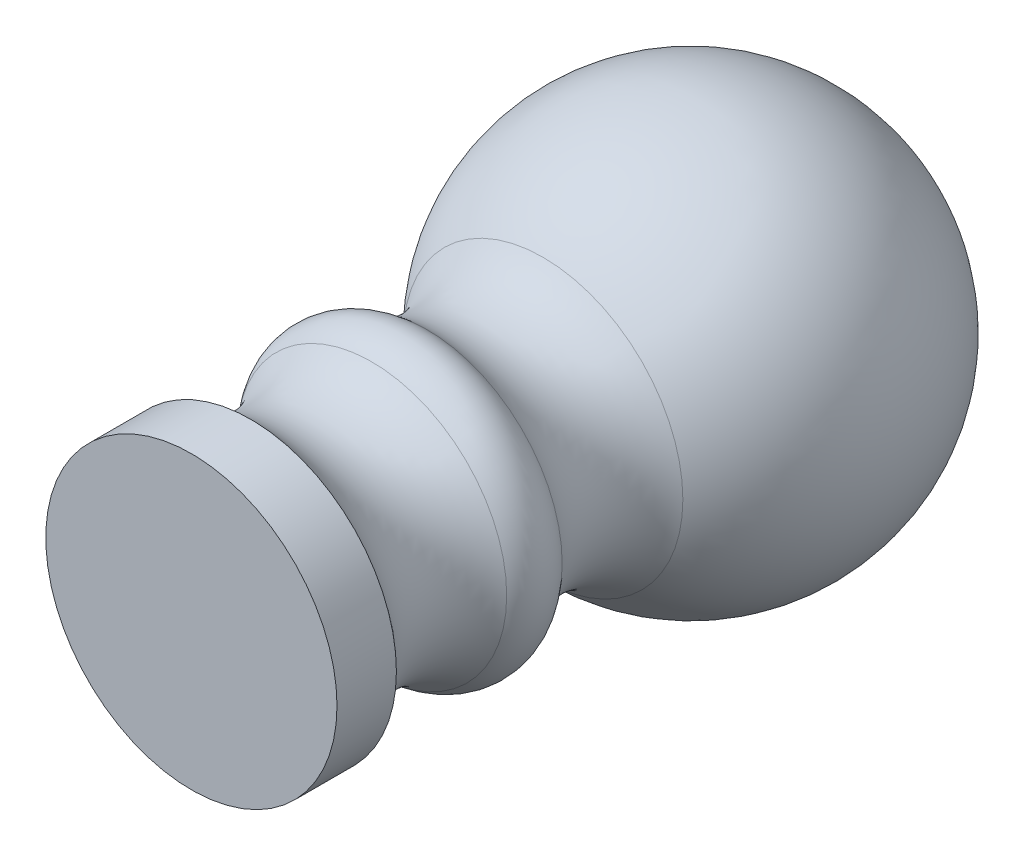
ISO-10303-21;
HEADER;
FILE_DESCRIPTION(('STEP AP214'),'2;1');
FILE_NAME('part.step','',(''),(''),'','','');
FILE_SCHEMA(('AUTOMOTIVE_DESIGN { 1 0 10303 214 1 1 1 1 }'));
ENDSEC;
DATA;
#1=APPLICATION_CONTEXT('core data for automotive mechanical design processes');
#2=APPLICATION_PROTOCOL_DEFINITION('international standard','automotive_design',2000,#1);
#3=PRODUCT_CONTEXT('',#1,'mechanical');
#4=PRODUCT('Part','Part','',(#3));
#5=PRODUCT_RELATED_PRODUCT_CATEGORY('part','',(#4));
#6=PRODUCT_DEFINITION_FORMATION('','',#4);
#7=PRODUCT_DEFINITION_CONTEXT('part definition',#1,'design');
#8=PRODUCT_DEFINITION('design','',#6,#7);
#9=PRODUCT_DEFINITION_SHAPE('','',#8);
#10=(LENGTH_UNIT() NAMED_UNIT(*) SI_UNIT(.MILLI.,.METRE.));
#11=(NAMED_UNIT(*) PLANE_ANGLE_UNIT() SI_UNIT($,.RADIAN.));
#12=(NAMED_UNIT(*) SI_UNIT($,.STERADIAN.) SOLID_ANGLE_UNIT());
#13=UNCERTAINTY_MEASURE_WITH_UNIT(LENGTH_MEASURE(1.E-05),#10,'distance_accuracy_value','');
#14=(GEOMETRIC_REPRESENTATION_CONTEXT(3) GLOBAL_UNCERTAINTY_ASSIGNED_CONTEXT((#13)) GLOBAL_UNIT_ASSIGNED_CONTEXT((#10,
#11,#12)) REPRESENTATION_CONTEXT('',''));
#15=CARTESIAN_POINT('',(0.,0.,0.));
#16=DIRECTION('',(0.,0.,1.));
#17=DIRECTION('',(1.,0.,0.));
#18=AXIS2_PLACEMENT_3D('',#15,#16,#17);
#19=CARTESIAN_POINT('',(0.,0.,-24.));
#20=DIRECTION('',(0.,0.,1.));
#21=DIRECTION('',(1.,0.,0.));
#22=AXIS2_PLACEMENT_3D('',#19,#20,#21);
#23=SPHERICAL_SURFACE('',#22,9.77393769225038);
#24=CARTESIAN_POINT('',(-8.91795144705289,0.,-24.));
#25=DIRECTION('',(1.,0.,0.));
#26=DIRECTION('',(0.,0.,-1.));
#27=AXIS2_PLACEMENT_3D('',#24,#25,#26);
#28=CIRCLE('',#27,4.);
#29=CARTESIAN_POINT('',(-8.91795144705289,0.,-28.));
#30=VERTEX_POINT('',#29);
#31=EDGE_CURVE('E45',#30,#30,#28,.T.);
#32=ORIENTED_EDGE('',*,*,#31,.T.);
#33=EDGE_LOOP('',(#32));
#34=FACE_BOUND('',#33,.T.);
#35=CARTESIAN_POINT('',(0.,0.,-16.9040352071946));
#36=DIRECTION('',(0.,0.,1.));
#37=DIRECTION('',(1.,0.,0.));
#38=AXIS2_PLACEMENT_3D('',#35,#36,#37);
#39=CIRCLE('',#38,6.72139432493431);
#40=CARTESIAN_POINT('',(6.72139432493431,0.,-16.9040352071946));
#41=VERTEX_POINT('',#40);
#42=EDGE_CURVE('E106',#41,#41,#39,.T.);
#43=ORIENTED_EDGE('',*,*,#42,.F.);
#44=EDGE_LOOP('',(#43));
#45=FACE_BOUND('',#44,.T.);
#46=CARTESIAN_POINT('',(0.,-8.91795144705289,-24.));
#47=DIRECTION('',(0.,1.,0.));
#48=DIRECTION('',(0.,0.,1.));
#49=AXIS2_PLACEMENT_3D('',#46,#47,#48);
#50=CIRCLE('',#49,4.);
#51=CARTESIAN_POINT('',(0.,-8.91795144705289,-20.));
#52=VERTEX_POINT('',#51);
#53=EDGE_CURVE('E100',#52,#52,#50,.T.);
#54=ORIENTED_EDGE('',*,*,#53,.T.);
#55=EDGE_LOOP('',(#54));
#56=FACE_BOUND('',#55,.T.);
#57=ADVANCED_FACE('F39',(#34,#45,#56),#23,.T.);
#58=CARTESIAN_POINT('',(4.,0.,-24.));
#59=DIRECTION('',(-1.,0.,0.));
#60=DIRECTION('',(0.,0.,1.));
#61=AXIS2_PLACEMENT_3D('',#58,#59,#60);
#62=CYLINDRICAL_SURFACE('',#61,4.);
#63=ORIENTED_EDGE('',*,*,#31,.F.);
#64=EDGE_LOOP('',(#63));
#65=FACE_BOUND('',#64,.T.);
#66=CARTESIAN_POINT('',(0.,0.,-24.));
#67=DIRECTION('',(-0.707106781186547,0.707106781186547,0.));
#68=DIRECTION('',(-0.707106781186547,-0.707106781186547,0.));
#69=AXIS2_PLACEMENT_3D('',#66,#67,#68);
#70=ELLIPSE('',#69,5.65685424949238,4.);
#71=CARTESIAN_POINT('',(0.,0.,-20.));
#72=VERTEX_POINT('',#71);
#73=CARTESIAN_POINT('',(0.,0.,-28.));
#74=VERTEX_POINT('',#73);
#75=EDGE_CURVE('E53',#72,#74,#70,.F.);
#76=ORIENTED_EDGE('',*,*,#75,.T.);
#77=CARTESIAN_POINT('',(0.,0.,-24.));
#78=DIRECTION('',(-0.707106781186547,-0.707106781186547,0.));
#79=DIRECTION('',(-0.707106781186547,0.707106781186547,0.));
#80=AXIS2_PLACEMENT_3D('',#77,#78,#79);
#81=ELLIPSE('',#80,5.65685424949238,4.);
#82=CARTESIAN_POINT('',(-4.,4.,-24.));
#83=VERTEX_POINT('',#82);
#84=EDGE_CURVE('E79',#74,#83,#81,.F.);
#85=ORIENTED_EDGE('',*,*,#84,.T.);
#86=EDGE_CURVE('E87',#83,#72,#81,.F.);
#87=ORIENTED_EDGE('',*,*,#86,.T.);
#88=EDGE_LOOP('',(#76,#85,#87));
#89=FACE_BOUND('',#88,.T.);
#90=ADVANCED_FACE('F142',(#65,#89),#62,.F.);
#91=CARTESIAN_POINT('',(0.,0.,0.));
#92=DIRECTION('',(0.,0.,1.));
#93=DIRECTION('',(1.,0.,0.));
#94=AXIS2_PLACEMENT_3D('',#91,#92,#93);
#95=PLANE('',#94);
#96=CARTESIAN_POINT('',(0.,0.,0.));
#97=DIRECTION('',(0.,0.,1.));
#98=DIRECTION('',(1.,0.,0.));
#99=AXIS2_PLACEMENT_3D('',#96,#97,#98);
#100=CIRCLE('',#99,7.);
#101=CARTESIAN_POINT('',(7.,0.,0.));
#102=VERTEX_POINT('',#101);
#103=EDGE_CURVE('E11',#102,#102,#100,.T.);
#104=ORIENTED_EDGE('',*,*,#103,.T.);
#105=EDGE_LOOP('',(#104));
#106=FACE_BOUND('',#105,.T.);
#107=ADVANCED_FACE('F150',(#106),#95,.T.);
#108=CARTESIAN_POINT('',(0.,0.,0.));
#109=DIRECTION('',(0.,0.,1.));
#110=DIRECTION('',(1.,0.,0.));
#111=AXIS2_PLACEMENT_3D('',#108,#109,#110);
#112=CYLINDRICAL_SURFACE('',#111,7.);
#113=CARTESIAN_POINT('',(0.,0.,-2.85539448897031));
#114=DIRECTION('',(0.,0.,1.));
#115=DIRECTION('',(1.,0.,0.));
#116=AXIS2_PLACEMENT_3D('',#113,#114,#115);
#117=CIRCLE('',#116,7.);
#118=CARTESIAN_POINT('',(7.,0.,-2.85539448897031));
#119=VERTEX_POINT('',#118);
#120=EDGE_CURVE('E50',#119,#119,#117,.T.);
#121=ORIENTED_EDGE('',*,*,#120,.T.);
#122=EDGE_LOOP('',(#121));
#123=FACE_BOUND('',#122,.T.);
#124=ORIENTED_EDGE('',*,*,#103,.F.);
#125=EDGE_LOOP('',(#124));
#126=FACE_BOUND('',#125,.T.);
#127=ADVANCED_FACE('F122',(#123,#126),#112,.T.);
#128=CARTESIAN_POINT('',(0.,0.,-6.));
#129=DIRECTION('',(0.,0.,1.));
#130=DIRECTION('',(1.,0.,0.));
#131=AXIS2_PLACEMENT_3D('',#128,#129,#130);
#132=TOROIDAL_SURFACE('',#131,9.47213595499958,4.);
#133=ORIENTED_EDGE('',*,*,#120,.F.);
#134=EDGE_LOOP('',(#133));
#135=FACE_BOUND('',#134,.T.);
#136=CARTESIAN_POINT('',(0.,0.,-8.66666666666667));
#137=DIRECTION('',(0.,0.,1.));
#138=DIRECTION('',(1.,0.,0.));
#139=AXIS2_PLACEMENT_3D('',#136,#137,#138);
#140=CIRCLE('',#139,6.49071198499986);
#141=CARTESIAN_POINT('',(6.49071198499986,0.,-8.66666666666667));
#142=VERTEX_POINT('',#141);
#143=EDGE_CURVE('E113',#142,#142,#140,.T.);
#144=ORIENTED_EDGE('',*,*,#143,.T.);
#145=EDGE_LOOP('',(#144));
#146=FACE_BOUND('',#145,.T.);
#147=ADVANCED_FACE('F124',(#135,#146),#132,.F.);
#148=CARTESIAN_POINT('',(0.,0.,-10.));
#149=DIRECTION('',(0.,0.,1.));
#150=DIRECTION('',(1.,0.,0.));
#151=AXIS2_PLACEMENT_3D('',#148,#149,#150);
#152=TOROIDAL_SURFACE('',#151,5.,2.);
#153=CARTESIAN_POINT('',(0.,0.,-11.3333333333333));
#154=DIRECTION('',(0.,0.,1.));
#155=DIRECTION('',(1.,0.,0.));
#156=AXIS2_PLACEMENT_3D('',#153,#154,#155);
#157=CIRCLE('',#156,6.49071198499986);
#158=CARTESIAN_POINT('',(6.49071198499986,0.,-11.3333333333333));
#159=VERTEX_POINT('',#158);
#160=EDGE_CURVE('E115',#159,#159,#157,.T.);
#161=ORIENTED_EDGE('',*,*,#160,.T.);
#162=EDGE_LOOP('',(#161));
#163=FACE_BOUND('',#162,.T.);
#164=ORIENTED_EDGE('',*,*,#143,.F.);
#165=EDGE_LOOP('',(#164));
#166=FACE_BOUND('',#165,.T.);
#167=ADVANCED_FACE('F130',(#163,#166),#152,.T.);
#168=CARTESIAN_POINT('',(0.,0.,-14.));
#169=DIRECTION('',(0.,0.,1.));
#170=DIRECTION('',(1.,0.,0.));
#171=AXIS2_PLACEMENT_3D('',#168,#169,#170);
#172=TOROIDAL_SURFACE('',#171,9.47213595499958,4.);
#173=ORIENTED_EDGE('',*,*,#160,.F.);
#174=EDGE_LOOP('',(#173));
#175=FACE_BOUND('',#174,.T.);
#176=ORIENTED_EDGE('',*,*,#42,.T.);
#177=EDGE_LOOP('',(#176));
#178=FACE_BOUND('',#177,.T.);
#179=ADVANCED_FACE('F132',(#175,#178),#172,.F.);
#180=CARTESIAN_POINT('',(0.,4.,-24.));
#181=DIRECTION('',(0.,-1.,0.));
#182=DIRECTION('',(0.,0.,-1.));
#183=AXIS2_PLACEMENT_3D('',#180,#181,#182);
#184=CYLINDRICAL_SURFACE('',#183,4.);
#185=ORIENTED_EDGE('',*,*,#53,.F.);
#186=EDGE_LOOP('',(#185));
#187=FACE_BOUND('',#186,.T.);
#188=CARTESIAN_POINT('',(0.,0.,-24.));
#189=DIRECTION('',(-0.707106781186547,-0.707106781186547,0.));
#190=DIRECTION('',(-0.707106781186547,0.707106781186547,0.));
#191=AXIS2_PLACEMENT_3D('',#188,#189,#190);
#192=ELLIPSE('',#191,5.65685424949238,4.);
#193=CARTESIAN_POINT('',(4.,-4.,-24.));
#194=VERTEX_POINT('',#193);
#195=EDGE_CURVE('E85',#194,#72,#192,.T.);
#196=ORIENTED_EDGE('',*,*,#195,.F.);
#197=EDGE_CURVE('E101',#74,#194,#192,.T.);
#198=ORIENTED_EDGE('',*,*,#197,.F.);
#199=ORIENTED_EDGE('',*,*,#75,.F.);
#200=EDGE_LOOP('',(#196,#198,#199));
#201=FACE_BOUND('',#200,.T.);
#202=ADVANCED_FACE('F138',(#187,#201),#184,.F.);
#203=CARTESIAN_POINT('',(4.,0.,-24.));
#204=DIRECTION('',(1.,0.,0.));
#205=DIRECTION('',(0.,0.,-1.));
#206=AXIS2_PLACEMENT_3D('',#203,#204,#205);
#207=PLANE('',#206);
#208=CARTESIAN_POINT('',(4.,0.,-24.));
#209=DIRECTION('',(1.,0.,0.));
#210=DIRECTION('',(0.,0.,-1.));
#211=AXIS2_PLACEMENT_3D('',#208,#209,#210);
#212=CIRCLE('',#211,4.);
#213=CARTESIAN_POINT('',(4.,4.,-24.));
#214=VERTEX_POINT('',#213);
#215=EDGE_CURVE('E97',#194,#214,#212,.T.);
#216=ORIENTED_EDGE('',*,*,#215,.F.);
#217=EDGE_CURVE('E96',#214,#194,#212,.T.);
#218=ORIENTED_EDGE('',*,*,#217,.F.);
#219=EDGE_LOOP('',(#216,#218));
#220=FACE_BOUND('',#219,.T.);
#221=ADVANCED_FACE('F102',(#220),#207,.F.);
#222=CARTESIAN_POINT('',(0.,0.,-24.));
#223=DIRECTION('',(-0.707106781186547,0.707106781186547,0.));
#224=DIRECTION('',(-0.707106781186547,-0.707106781186547,0.));
#225=AXIS2_PLACEMENT_3D('',#222,#223,#224);
#226=ELLIPSE('',#225,5.65685424949238,4.);
#227=EDGE_CURVE('E74',#214,#74,#226,.T.);
#228=ORIENTED_EDGE('',*,*,#227,.T.);
#229=ORIENTED_EDGE('',*,*,#197,.T.);
#230=ORIENTED_EDGE('',*,*,#215,.T.);
#231=EDGE_LOOP('',(#228,#229,#230));
#232=FACE_BOUND('',#231,.T.);
#233=ADVANCED_FACE('F99',(#232),#62,.F.);
#234=ORIENTED_EDGE('',*,*,#195,.T.);
#235=EDGE_CURVE('E62',#72,#214,#226,.T.);
#236=ORIENTED_EDGE('',*,*,#235,.T.);
#237=ORIENTED_EDGE('',*,*,#217,.T.);
#238=EDGE_LOOP('',(#234,#236,#237));
#239=FACE_BOUND('',#238,.T.);
#240=ADVANCED_FACE('F94',(#239),#62,.F.);
#241=ORIENTED_EDGE('',*,*,#227,.F.);
#242=CARTESIAN_POINT('',(0.,4.,-24.));
#243=DIRECTION('',(0.,1.,0.));
#244=DIRECTION('',(0.,0.,1.));
#245=AXIS2_PLACEMENT_3D('',#242,#243,#244);
#246=CIRCLE('',#245,4.);
#247=EDGE_CURVE('E77',#214,#83,#246,.T.);
#248=ORIENTED_EDGE('',*,*,#247,.T.);
#249=ORIENTED_EDGE('',*,*,#84,.F.);
#250=EDGE_LOOP('',(#241,#248,#249));
#251=FACE_BOUND('',#250,.T.);
#252=ADVANCED_FACE('F73',(#251),#184,.F.);
#253=CARTESIAN_POINT('',(0.,4.,-24.));
#254=DIRECTION('',(0.,1.,0.));
#255=DIRECTION('',(0.,0.,1.));
#256=AXIS2_PLACEMENT_3D('',#253,#254,#255);
#257=PLANE('',#256);
#258=EDGE_CURVE('E81',#83,#214,#246,.T.);
#259=ORIENTED_EDGE('',*,*,#258,.F.);
#260=ORIENTED_EDGE('',*,*,#247,.F.);
#261=EDGE_LOOP('',(#259,#260));
#262=FACE_BOUND('',#261,.T.);
#263=ADVANCED_FACE('F89',(#262),#257,.F.);
#264=ORIENTED_EDGE('',*,*,#86,.F.);
#265=ORIENTED_EDGE('',*,*,#258,.T.);
#266=ORIENTED_EDGE('',*,*,#235,.F.);
#267=EDGE_LOOP('',(#264,#265,#266));
#268=FACE_BOUND('',#267,.T.);
#269=ADVANCED_FACE('F88',(#268),#184,.F.);
#270=CLOSED_SHELL('',(#57,#90,#107,#127,#147,#167,#179,#202,#221,#233,#240,#252,#263,#269));
#271=MANIFOLD_SOLID_BREP('B2',#270);
#272=ADVANCED_BREP_SHAPE_REPRESENTATION('',(#18,#271),#14);
#273=SHAPE_DEFINITION_REPRESENTATION(#9,#272);
ENDSEC;
END-ISO-10303-21;
